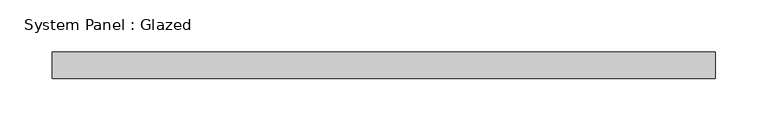
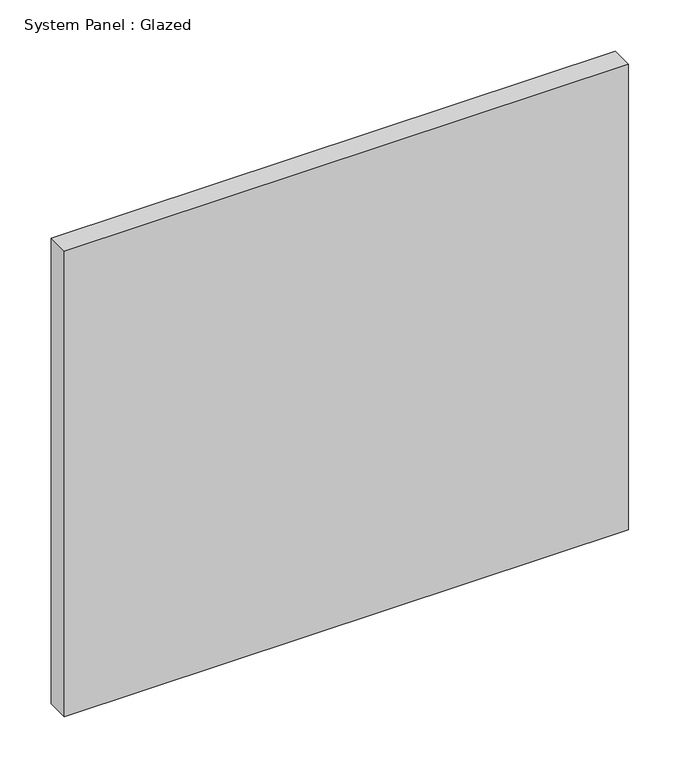
"""IFC4 building model written with IfcOpenShell, lengths in millimetres: plate geometry, System Panel : Glazed."""

from ifc_helpers import new_model, si_unit, origin, origin_with_axes, place, context, project, spatial, polyline, outline, extrude, source, transform, mapped, element, save


def system_panel_glazed_8c040c01(model_context):
    return source(origin(), model_context, "Body", "SweptSolid", [
        extrude(outline(polyline([(317.5, 19.05), (-317.5, 19.05), (-317.5, 44.45), (317.5, 44.45), (317.5, 19.05)])), origin_with_axes(), (0.0, 0.0, 1.0), 553.7348788),
    ])


if __name__ == "__main__":
    model = new_model("IFC4")
    model_context = context("Model", 3, world=origin())
    ifc_project = project(units=[si_unit("LENGTHUNIT", "METRE", prefix="MILLI")], contexts=[model_context])
    site = spatial("IfcSite", under=ifc_project)
    building = spatial("IfcBuilding", under=site)
    placement = place(None, origin())
    system_panel_glazed_shape = system_panel_glazed_8c040c01(model_context)
    element("IfcPlate", 1, ObjectType="System Panel : Glazed", at=placement, inside=building, context=model_context, shape_type="MappedRepresentation", body=[
        mapped(system_panel_glazed_shape, transform((0.0, 0.0, 0.0), x_axis=(1.0, 0.0, 0.0), y_axis=(0.0, 1.0, 0.0), z_axis=(0.0, 0.0, 1.0))),
    ])
    save(model, "model.ifc")

# Revit data of these elements
# Type "System Panel : Glazed"
#   Construction Type Id = "GSP4R"
#   Analytic Construction = "1/8 in Pilkington single glazing"
#   Visual Light Transmittance = 0.9
#   Solar Heat Gain Coefficient = 0.86
#   Heat Transfer Coefficient (U) = 1.18115 BTU/(h·ft²·°F)
#   Define Thermal Properties by = 1
# Element 1 (IfcPlate, "System Panel : Glazed")
#   Materials on its faces: "Glass"
# Materials
#   "Glass": class "Glass", colour RGB 0 128 192, transparency 0.75, Description = "Soda Lime Glass", Cost = 0
